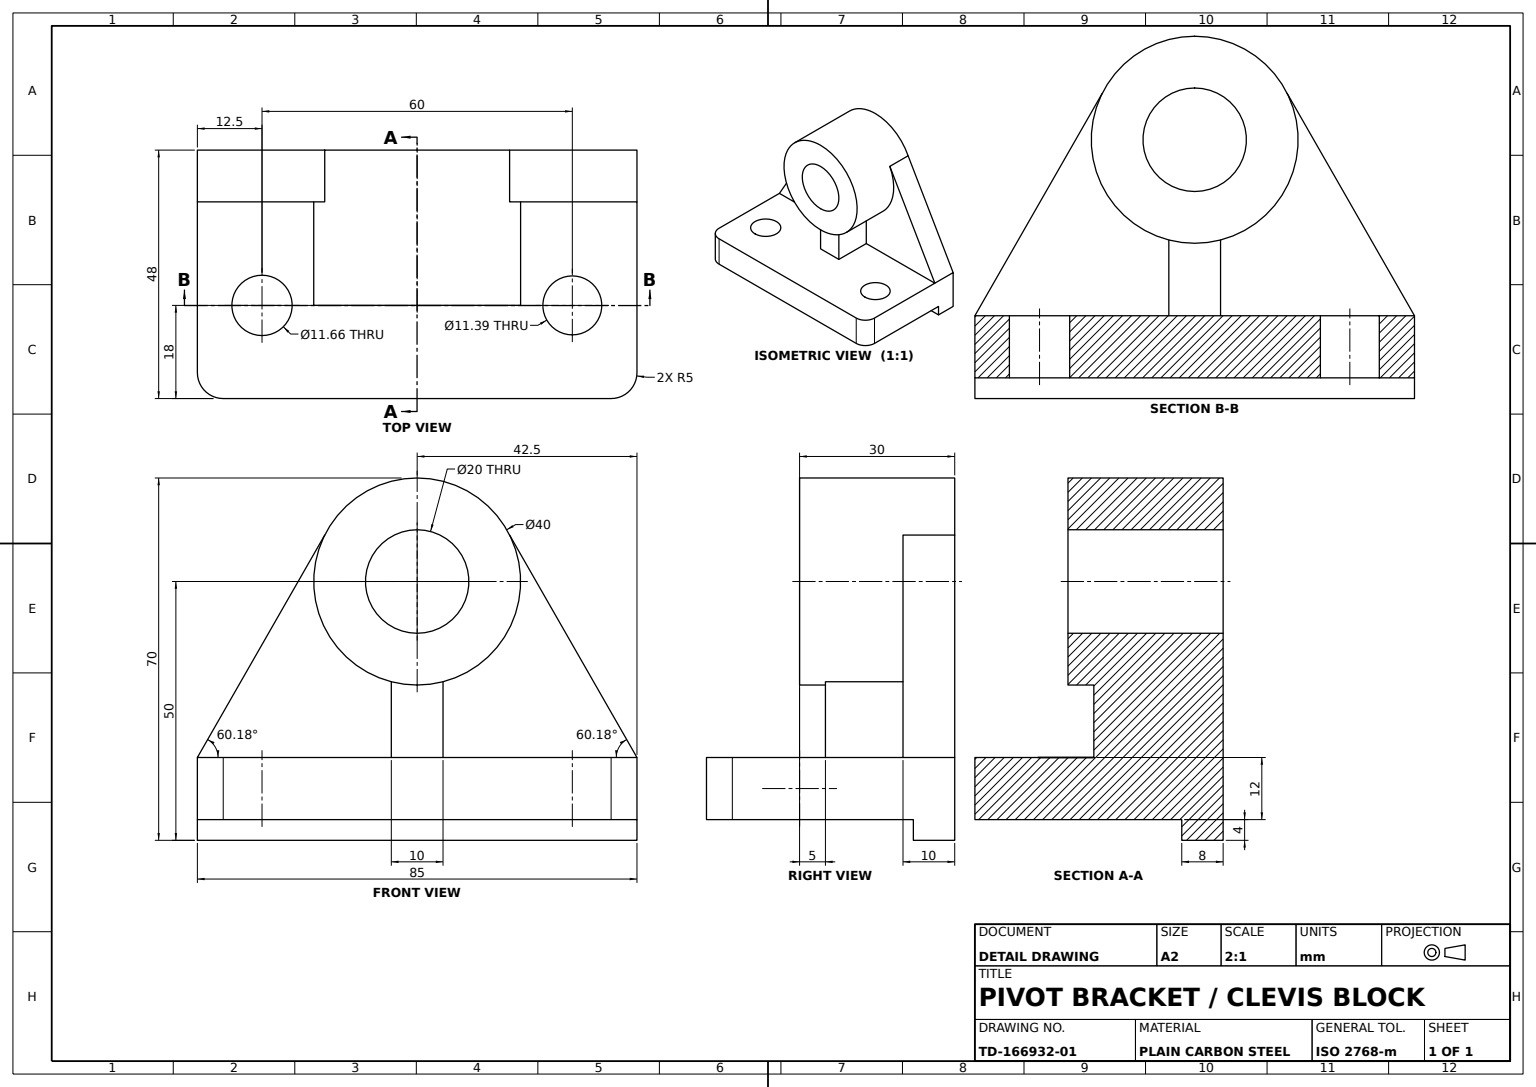
from build123d import *

# Parameters (mm, degrees)
BASE_PLATE_DEPTH              = 85
PIVOT_BOSS_SKETCH_R           = 20
PIVOT_BOSS_DEPTH              = 30
GUSSET_RIB_DEPTH              = 10
BOSS_SUPPORT_BLOCK_REACH      = 113.557
BOSS_SUPPORT_BLOCK_END_RADIUS = 20
BOSS_SUPPORT_BLOCK_SKETCH_W   = 15
BOSS_SUPPORT_BLOCK_SKETCH_H   = 10
PIVOT_BORE_SKETCH_R           = 10
PIVOT_BORE_20_DEPTH           = 115.127122105
MOUNTING_HOLES_SKETCH_R       = 5.697054252
MOUNTING_HOLES_SKETCH_R_2     = 5.829543886
MOUNTING_HOLES_2X_DEPTH       = 112.557160236
CORNER_FILLETS_R5_R           = 5


with BuildPart() as part:
    # Base Plate Profile Sketch → Base Plate (new body)
    with BuildSketch(Plane.XY):
        Polygon((0, 0), (0, 16), (48, 16), (48, 4), (8, 4), (8, 0), align=None)
    extrude(amount=BASE_PLATE_DEPTH)



with BuildPart() as body_2:
    # Pivot Boss Sketch → Pivot Boss (new body)
    with BuildSketch(Plane.ZY):
        with Locations(Location((42.5, 50, 0), (0, 0, 270))):
            Circle(PIVOT_BOSS_SKETCH_R)
    extrude(amount=-PIVOT_BOSS_DEPTH)


with BuildPart() as part_1:
    add(part.part)

    add(body_2.part)  # Gusset Rib merges body 2
    # Gusset Rib Sketch → Gusset Rib (add)
    with BuildSketch(Plane.ZY):
        with BuildLine():
            Line((24.625908668, 58.973118691), (0, 16))
            Line((0, 16), (85, 16))
            Line((85, 16), (60.374091332, 58.973118691))
            ThreePointArc((60.374091332, 58.973118691), (61.961267002, 54.610757712), (62.5, 50))
            ThreePointArc((62.5, 50), (37.889242288, 30.538732998), (24.625908668, 58.973118691))
        make_face()
    extrude(amount=-GUSSET_RIB_DEPTH)

    # Boss Support Block: up to this cylinder (the profile starts outside it)
    boss_support_block_end = Plane(origin=(17.5, 50, 42.5), z_dir=(-1, 0, 0)) * Cylinder(BOSS_SUPPORT_BLOCK_END_RADIUS, 268.114, mode=Mode.PRIVATE)
    # Boss Support Block Sketch → Boss Support Block (add, up to the surface)
    with BuildSketch(Plane(origin=(0, 16, 0), x_dir=(1, 0, 0), z_dir=(0, 1, 0)), mode=Mode.PRIVATE) as boss_support_block_sk1:
        with Locations((17.5, -42.5)):
            Rectangle(BOSS_SUPPORT_BLOCK_SKETCH_W, BOSS_SUPPORT_BLOCK_SKETCH_H)
    boss_support_block_tool1 = extrude(boss_support_block_sk1.sketch, amount=BOSS_SUPPORT_BLOCK_REACH, mode=Mode.PRIVATE) - boss_support_block_end
    add(boss_support_block_tool1.solids().sort_by_distance((17.5, 16, 42.5))[0])

    # Pivot Bore Sketch → Pivot Bore Ø20 (cut, through all)
    with BuildSketch(Plane(origin=(30, 0, 0), x_dir=(0, 0, -1), z_dir=(1, 0, 0))):
        with Locations(Location((-42.5, 50, 0), (0, 0, 90))):
            Circle(PIVOT_BORE_SKETCH_R)
    extrude(amount=-PIVOT_BORE_20_DEPTH, mode=Mode.SUBTRACT)

    # Mounting Holes Sketch → Mounting Holes 2x (cut, through all)
    with BuildSketch(Plane(origin=(0, 16, 0), x_dir=(1, 0, 0), z_dir=(0, 1, 0))):
        with Locations(Location((30, -12.5, 0), (0, 0, 180))):
            Circle(MOUNTING_HOLES_SKETCH_R)
        with Locations(Location((30, -72.5, 0), (0, 0, 180))):
            Circle(MOUNTING_HOLES_SKETCH_R_2)
    extrude(amount=-MOUNTING_HOLES_2X_DEPTH, mode=Mode.SUBTRACT)

    # Corner Fillets R5
    corner_fillets_r5_edges = [part_1.edges().sort_by_distance(p)[0] for p in [
        (48, 10, 85),
        (48, 10, 0),
    ]]
    fillet(corner_fillets_r5_edges, radius=CORNER_FILLETS_R5_R)


solid = part_1.part
